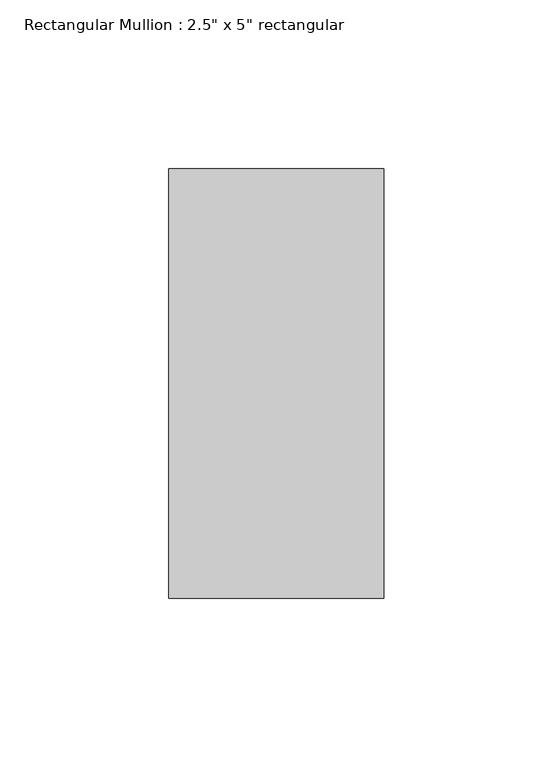
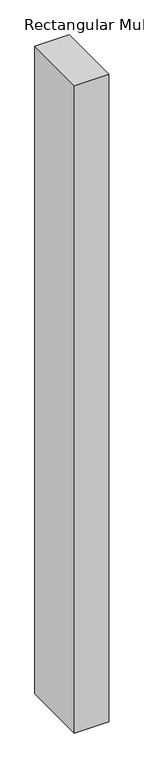
"""IFC4 building model written with IfcOpenShell, lengths in millimetres: member geometry."""

from ifc_helpers import new_model, si_unit, frame, origin, place, context, project, spatial, polyline, outline, extrude, source, transform, mapped, element, save


def member_d6537dc6(model_context):
    return source(origin(), model_context, "Body", "SweptSolid", [
        extrude(outline(polyline([(0.0, 63.5), (0.0, -63.5), (-63.5, -63.5), (-63.5, 63.5), (0.0, 63.5)])), frame((0.0, 0.0, -1269.895932), z_axis=(0.0, 0.0, 1.0), x_axis=(1.0, 0.0, 0.0)), (0.0, 0.0, 1.0), 1269.895932),
    ])


if __name__ == "__main__":
    model = new_model("IFC4")
    model_context = context("Model", 3, world=origin())
    ifc_project = project(units=[si_unit("LENGTHUNIT", "METRE", prefix="MILLI")], contexts=[model_context])
    site = spatial("IfcSite", under=ifc_project)
    building = spatial("IfcBuilding", under=site)
    placement = place(None, origin())
    member_shape = member_d6537dc6(model_context)
    element("IfcMember", 1, ObjectType="Rectangular Mullion : 2.5\" x 5\" rectangular", at=placement, inside=building, context=model_context, shape_type="MappedRepresentation", body=[
        mapped(member_shape, transform((0.0, 0.0, 0.0), x_axis=(1.0, 0.0, 0.0), y_axis=(0.0, 1.0, 0.0), z_axis=(0.0, 0.0, 1.0))),
    ])
    save(model, "model.ifc")

# Revit data of these elements
# Type "Rectangular Mullion : 2.5\" x 5\" rectangular"
#   built-in parameter 1007304 = 0.416667 (stored number, unit not read)
#   built-in parameter 1007301 = 0.104167 (stored number, unit not read)
#   built-in parameter 1007300 = 0.104167 (stored number, unit not read)
# Element 1 (IfcMember, "Rectangular Mullion : 2.5\" x 5\" rectangular")
#   Materials on its faces: "Aluminum"
# Materials
#   "Aluminum": class "Metal", colour RGB 247 247 247, transparency 0, Description = "Aluminum 6061", Cost = 0
